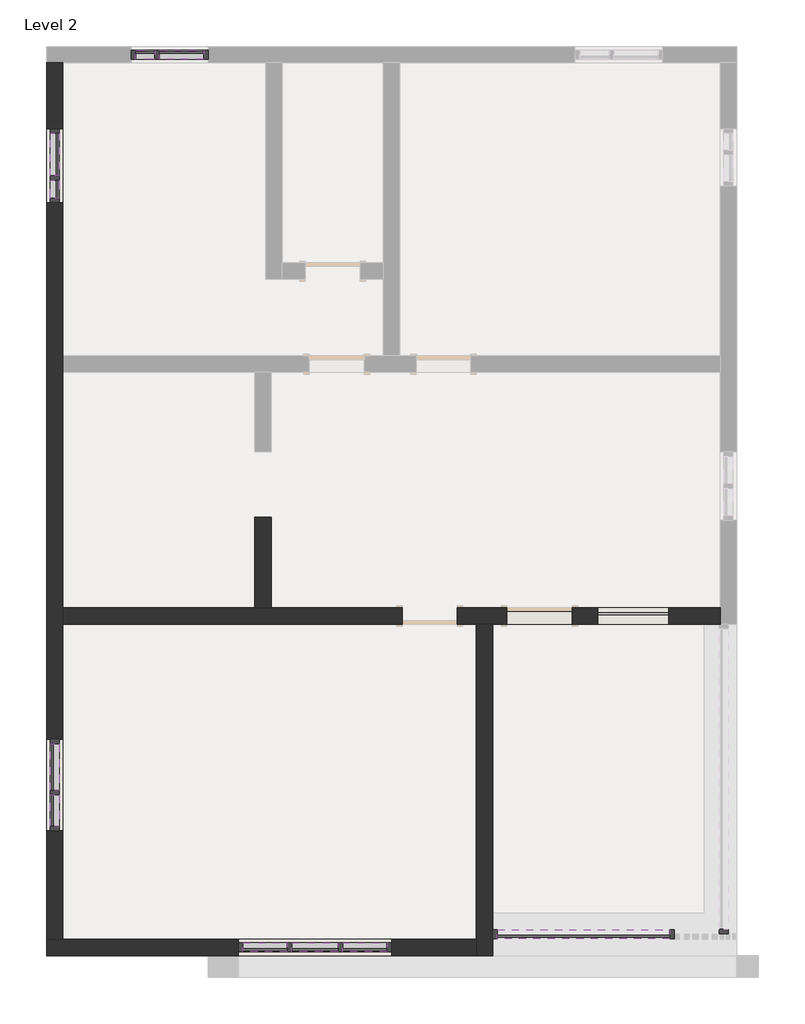
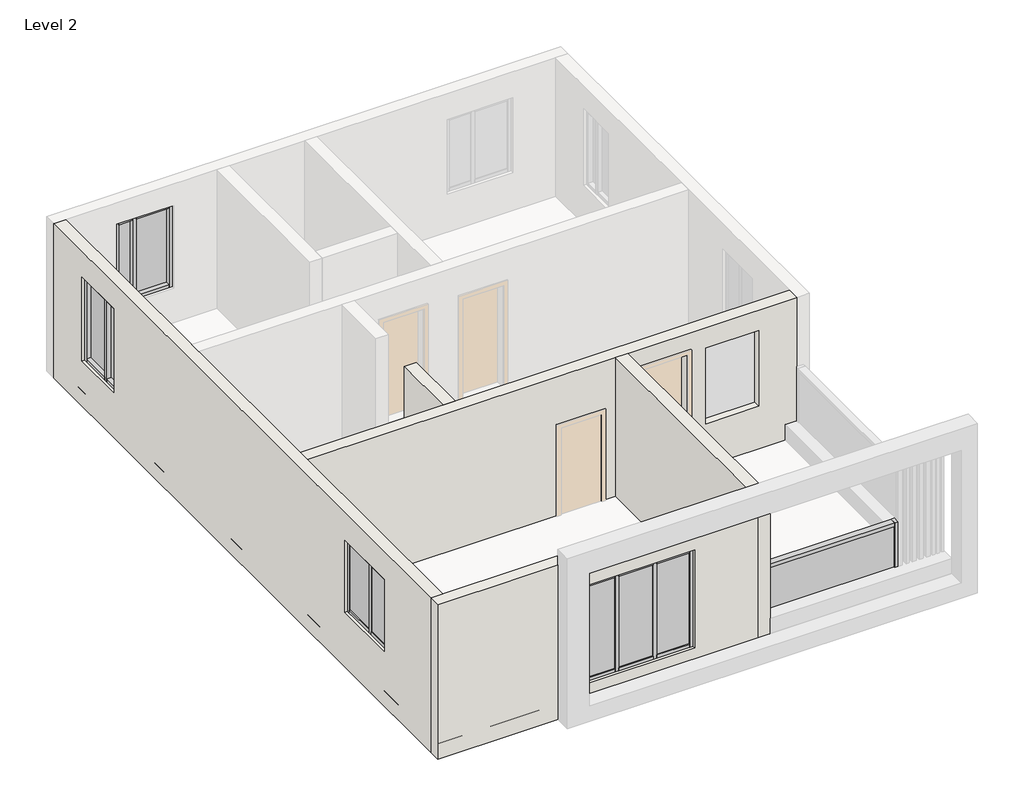
# One storey, part 1 of 2: 36 members, 10 plates, 5 walls.
"""IFC4 building model written with IfcOpenShell, lengths in millimetres."""

from ifc_helpers import new_model, si_unit, frame, origin, place, context, project, spatial, polyline, outline, extrude, faceted_brep, transform, mapped, element, save
from components import member_6fb4a552, member_e5d39754, member_3f0e0172, member_c304ec9f, member_9857a5fa, member_5215b92c, member_4adcbd6e, member_2f7568ae, member_e2524bce, member_4d06fd9b, member_4c0b5a72, member_ac37c43a, member_5cae1c76, member_8a84510b, member_26f0793c, member_c92b576d, member_86c371d5, member_6146d365, system_panel_glazed_d2c96357, system_panel_glazed_1c0d1104, system_panel_glazed_012e7337, system_panel_glazed_f6599d2c, system_panel_glazed_978b3bbc, system_panel_glazed_5a7f8ff5, system_panel_glazed_b38058b2, system_panel_glazed_fafcfa65, system_panel_glazed_51b229ca

model = new_model("IFC4")

# Units and contexts
model_context = context("Model", 3, world=origin())
ifc_project = project(units=[si_unit("LENGTHUNIT", "METRE", prefix="MILLI")], contexts=[model_context])

# Site, building, storey
site = spatial("IfcSite", under=ifc_project)
building = spatial("IfcBuilding", under=site)
storey = spatial("IfcBuildingStorey", under=building, Name="Level 2", Elevation=3048.0)

# Members
placement = place(None, origin())
member_shape = member_6fb4a552(model_context)
element("IfcMember", 1, ObjectType="Rectangular Mullion : 2.5\" x 5\" rectangular", at=placement, inside=storey, context=model_context, shape_type="MappedRepresentation", body=[
    mapped(member_shape, transform((-18412.7628107, -12019.2142965, 4124.9991955), x_axis=(0.0, 0.0, -1.0), y_axis=(1.0, 0.0, 0.0), z_axis=(0.0, -1.0, 0.0))),
])
member_2_shape = member_e5d39754(model_context)
element("IfcMember", 2, ObjectType="Rectangular Mullion : 2.5\" x 5\" rectangular", at=placement, inside=storey, context=model_context, shape_type="MappedRepresentation", body=[
    mapped(member_2_shape, transform((-18412.7628107, -2373.5642965, 3937.6338928), x_axis=(0.0, 0.0, -1.0), y_axis=(-1.0, 0.0, 0.0), z_axis=(0.0, 1.0, 0.0))),
])
element("IfcMember", 3, ObjectType="Rectangular Mullion : 2.5\" x 5\" rectangular", at=placement, inside=storey, context=model_context, shape_type="MappedRepresentation", body=[
    mapped(member_shape, transform((-18412.7628107, -11581.0642965, 5550.0097681), x_axis=(0.0, 0.0, 1.0), y_axis=(1.0, 0.0, 0.0), z_axis=(0.0, 1.0, 0.0))),
])
element("IfcMember", 4, ObjectType="Rectangular Mullion : 2.5\" x 5\" rectangular", at=placement, inside=storey, context=model_context, shape_type="MappedRepresentation", body=[
    mapped(member_2_shape, transform((-18412.7628107, -2964.1142965, 5597.0626061), x_axis=(0.0, 0.0, 1.0), y_axis=(-1.0, 0.0, 0.0), z_axis=(0.0, -1.0, 0.0))),
])
member_3_shape = member_3f0e0172(model_context)
element("IfcMember", 5, ObjectType="Rectangular Mullion : 2.5\" x 5\" rectangular", at=placement, inside=storey, context=model_context, shape_type="MappedRepresentation", body=[
    mapped(member_3_shape, transform((-14405.9128107, -13701.9642965, 5498.9031317), x_axis=(0.0, 0.0, 1.0), y_axis=(0.0, 1.0, 0.0), z_axis=(-1.0, 0.0, 0.0))),
])
element("IfcMember", 6, ObjectType="Rectangular Mullion : 2.5\" x 5\" rectangular", at=placement, inside=storey, context=model_context, shape_type="MappedRepresentation", body=[
    mapped(member_3_shape, transform((-15796.5628107, -13701.9642965, 5498.9031317), x_axis=(0.0, 0.0, 1.0), y_axis=(0.0, 1.0, 0.0), z_axis=(-1.0, 0.0, 0.0))),
])
element("IfcMember", 7, ObjectType="Rectangular Mullion : 2.5\" x 5\" rectangular", at=placement, inside=storey, context=model_context, shape_type="MappedRepresentation", body=[
    mapped(member_3_shape, transform((-16342.6628107, -1281.3642965, 5669.0676645), x_axis=(0.0, 0.0, 1.0), y_axis=(0.0, -1.0, 0.0), z_axis=(1.0, 0.0, 0.0))),
])
element("IfcMember", 8, ObjectType="Rectangular Mullion : 2.5\" x 5\" rectangular", at=placement, inside=storey, context=model_context, shape_type="MappedRepresentation", body=[
    mapped(member_3_shape, transform((-15180.6128107, -13701.9642965, 3567.7093947), x_axis=(0.0, 0.0, -1.0), y_axis=(0.0, 1.0, 0.0), z_axis=(1.0, 0.0, 0.0))),
])
element("IfcMember", 9, ObjectType="Rectangular Mullion : 2.5\" x 5\" rectangular", at=placement, inside=storey, context=model_context, shape_type="MappedRepresentation", body=[
    mapped(member_3_shape, transform((-13789.9628107, -13701.9642965, 3567.7093947), x_axis=(0.0, 0.0, -1.0), y_axis=(0.0, 1.0, 0.0), z_axis=(1.0, 0.0, 0.0))),
])
element("IfcMember", 10, ObjectType="Rectangular Mullion : 2.5\" x 5\" rectangular", at=placement, inside=storey, context=model_context, shape_type="MappedRepresentation", body=[
    mapped(member_3_shape, transform((-16958.6128107, -1281.3642965, 4034.7127427), x_axis=(0.0, 0.0, -1.0), y_axis=(0.0, -1.0, 0.0), z_axis=(-1.0, 0.0, 0.0))),
])
member_4_shape = member_c304ec9f(model_context)
element("IfcMember", 11, ObjectType="Rectangular Mullion : 2.5\" x 5\" rectangular", at=placement, inside=storey, context=model_context, shape_type="MappedRepresentation", body=[
    mapped(member_4_shape, transform((-15860.0628107, -13701.9642965, 3567.7093947), x_axis=(-1.0, 0.0, 0.0), y_axis=(0.0, 1.0, 0.0), z_axis=(0.0, 0.0, -1.0))),
])
element("IfcMember", 12, ObjectType="Rectangular Mullion : 2.5\" x 5\" rectangular", at=placement, inside=storey, context=model_context, shape_type="MappedRepresentation", body=[
    mapped(member_4_shape, transform((-13726.4628107, -13701.9642965, 5498.9031317), x_axis=(1.0, 0.0, 0.0), y_axis=(0.0, 1.0, 0.0), z_axis=(0.0, 0.0, 1.0))),
])
member_5_shape = member_9857a5fa(model_context)
element("IfcMember", 13, ObjectType="Rectangular Mullion : 2.5\" x 5\" rectangular", at=placement, inside=storey, context=model_context, shape_type="MappedRepresentation", body=[
    mapped(member_5_shape, transform((-15148.8628107, -13701.9642965, 3567.7093947), x_axis=(-1.0, 0.0, 0.0), y_axis=(0.0, 1.0, 0.0), z_axis=(0.0, 0.0, -1.0))),
])
element("IfcMember", 14, ObjectType="Rectangular Mullion : 2.5\" x 5\" rectangular", at=placement, inside=storey, context=model_context, shape_type="MappedRepresentation", body=[
    mapped(member_5_shape, transform((-14437.6628107, -13701.9642965, 3567.7093947), x_axis=(-1.0, 0.0, 0.0), y_axis=(0.0, 1.0, 0.0), z_axis=(0.0, 0.0, -1.0))),
])
member_6_shape = member_5215b92c(model_context)
element("IfcMember", 15, ObjectType="Rectangular Mullion : 2.5\" x 5\" rectangular", at=placement, inside=storey, context=model_context, shape_type="MappedRepresentation", body=[
    mapped(member_6_shape, transform((-15117.1128107, -13701.9642965, 5498.9031317), x_axis=(0.0, 0.0, 1.0), y_axis=(0.0, 1.0, 0.0), z_axis=(-1.0, 0.0, 0.0))),
])
element("IfcMember", 16, ObjectType="Rectangular Mullion : 2.5\" x 5\" rectangular", at=placement, inside=storey, context=model_context, shape_type="MappedRepresentation", body=[
    mapped(member_6_shape, transform((-18412.7628107, -10869.8642965, 5550.0097681), x_axis=(0.0, 0.0, 1.0), y_axis=(1.0, 0.0, 0.0), z_axis=(0.0, 1.0, 0.0))),
])
element("IfcMember", 17, ObjectType="Rectangular Mullion : 2.5\" x 5\" rectangular", at=placement, inside=storey, context=model_context, shape_type="MappedRepresentation", body=[
    mapped(member_6_shape, transform((-14469.4128107, -13701.9642965, 3567.7093947), x_axis=(0.0, 0.0, -1.0), y_axis=(0.0, 1.0, 0.0), z_axis=(1.0, 0.0, 0.0))),
])
element("IfcMember", 18, ObjectType="Rectangular Mullion : 2.5\" x 5\" rectangular", at=placement, inside=storey, context=model_context, shape_type="MappedRepresentation", body=[
    mapped(member_6_shape, transform((-18412.7628107, -11517.5642965, 4124.9991955), x_axis=(0.0, 0.0, -1.0), y_axis=(1.0, 0.0, 0.0), z_axis=(0.0, -1.0, 0.0))),
])
member_7_shape = member_4adcbd6e(model_context)
element("IfcMember", 19, ObjectType="Rectangular Mullion : 2.5\" x 5\" rectangular", at=placement, inside=storey, context=model_context, shape_type="MappedRepresentation", body=[
    mapped(member_7_shape, transform((-17022.1128107, -1281.3642965, 5669.0676645), x_axis=(0.0, 0.0, 1.0), y_axis=(0.0, -1.0, 0.0), z_axis=(1.0, 0.0, 0.0))),
])
member_8_shape = member_2f7568ae(model_context)
element("IfcMember", 20, ObjectType="Rectangular Mullion : 2.5\" x 5\" rectangular", at=placement, inside=storey, context=model_context, shape_type="MappedRepresentation", body=[
    mapped(member_8_shape, transform((-16990.3628107, -1281.3642965, 4034.7127427), x_axis=(1.0, 0.0, 0.0), y_axis=(0.0, -1.0, 0.0), z_axis=(0.0, 0.0, -1.0))),
])
element("IfcMember", 21, ObjectType="Rectangular Mullion : 2.5\" x 5\" rectangular", at=placement, inside=storey, context=model_context, shape_type="MappedRepresentation", body=[
    mapped(member_7_shape, transform((-17282.4628107, -1281.3642965, 4034.7127427), x_axis=(0.0, 0.0, -1.0), y_axis=(0.0, -1.0, 0.0), z_axis=(-1.0, 0.0, 0.0))),
])
member_9_shape = member_e2524bce(model_context)
element("IfcMember", 22, ObjectType="Rectangular Mullion : 2.5\" x 5\" rectangular", at=placement, inside=storey, context=model_context, shape_type="MappedRepresentation", body=[
    mapped(member_9_shape, transform((-17345.9628107, -1281.3642965, 5669.0676645), x_axis=(-1.0, 0.0, 0.0), y_axis=(0.0, -1.0, 0.0), z_axis=(0.0, 0.0, 1.0))),
])
element("IfcMember", 23, ObjectType="Rectangular Mullion : 2.5\" x 5\" rectangular", at=placement, inside=storey, context=model_context, shape_type="MappedRepresentation", body=[
    mapped(member_9_shape, transform((-16279.1628107, -1281.3642965, 4034.7127427), x_axis=(1.0, 0.0, 0.0), y_axis=(0.0, -1.0, 0.0), z_axis=(0.0, 0.0, -1.0))),
])
member_10_shape = member_4d06fd9b(model_context)
element("IfcMember", 24, ObjectType="Rectangular Mullion : 2.5\" x 5\" rectangular", at=placement, inside=storey, context=model_context, shape_type="MappedRepresentation", body=[
    mapped(member_10_shape, transform((-18412.7628107, -3275.2642965, 5597.0626061), x_axis=(0.0, 0.0, 1.0), y_axis=(-1.0, 0.0, 0.0), z_axis=(0.0, -1.0, 0.0))),
])
member_11_shape = member_4c0b5a72(model_context)
element("IfcMember", 25, ObjectType="Rectangular Mullion : 2.5\" x 5\" rectangular", at=placement, inside=storey, context=model_context, shape_type="MappedRepresentation", body=[
    mapped(member_11_shape, transform((-18412.7628107, -2995.8642965, 3937.6338928), x_axis=(0.0, -1.0, 0.0), y_axis=(-1.0, 0.0, 0.0), z_axis=(0.0, 0.0, -1.0))),
])
element("IfcMember", 26, ObjectType="Rectangular Mullion : 2.5\" x 5\" rectangular", at=placement, inside=storey, context=model_context, shape_type="MappedRepresentation", body=[
    mapped(member_10_shape, transform((-18412.7628107, -3027.6142965, 3937.6338928), x_axis=(0.0, 0.0, -1.0), y_axis=(-1.0, 0.0, 0.0), z_axis=(0.0, 1.0, 0.0))),
])
member_12_shape = member_ac37c43a(model_context)
element("IfcMember", 27, ObjectType="Rectangular Mullion : 2.5\" x 5\" rectangular", at=placement, inside=storey, context=model_context, shape_type="MappedRepresentation", body=[
    mapped(member_12_shape, transform((-18412.7628107, -3338.7642965, 3937.6338928), x_axis=(0.0, -1.0, 0.0), y_axis=(-1.0, 0.0, 0.0), z_axis=(0.0, 0.0, -1.0))),
])
element("IfcMember", 28, ObjectType="Rectangular Mullion : 2.5\" x 5\" rectangular", at=placement, inside=storey, context=model_context, shape_type="MappedRepresentation", body=[
    mapped(member_12_shape, transform((-18412.7628107, -2310.0642965, 5597.0626061), x_axis=(0.0, 1.0, 0.0), y_axis=(-1.0, 0.0, 0.0), z_axis=(0.0, 0.0, 1.0))),
])
member_13_shape = member_5cae1c76(model_context)
element("IfcMember", 29, ObjectType="Rectangular Mullion : 2.5\" x 5\" rectangular", at=placement, inside=storey, context=model_context, shape_type="MappedRepresentation", body=[
    mapped(member_13_shape, transform((-18412.7628107, -11549.3142965, 4124.9991955), x_axis=(0.0, 1.0, 0.0), y_axis=(1.0, 0.0, 0.0), z_axis=(0.0, 0.0, -1.0))),
])
member_14_shape = member_8a84510b(model_context)
element("IfcMember", 30, ObjectType="Rectangular Mullion : 2.5\" x 5\" rectangular", at=placement, inside=storey, context=model_context, shape_type="MappedRepresentation", body=[
    mapped(member_14_shape, transform((-18412.7628107, -12082.7142965, 5550.0097681), x_axis=(0.0, -1.0, 0.0), y_axis=(1.0, 0.0, 0.0), z_axis=(0.0, 0.0, 1.0))),
])
element("IfcMember", 31, ObjectType="Rectangular Mullion : 2.5\" x 5\" rectangular", at=placement, inside=storey, context=model_context, shape_type="MappedRepresentation", body=[
    mapped(member_14_shape, transform((-18412.7628107, -10806.3642965, 4124.9991955), x_axis=(0.0, 1.0, 0.0), y_axis=(1.0, 0.0, 0.0), z_axis=(0.0, 0.0, -1.0))),
])
member_15_shape = member_26f0793c(model_context)
element("IfcMember", 32, ObjectType="Rectangular Mullion : 2.5\" x 5\" rectangular", at=placement, inside=storey, context=model_context, shape_type="MappedRepresentation", body=[
    mapped(member_15_shape, transform((-12316.7628107, -13518.1585678, 3513.341316), x_axis=(-1.0, 0.0, 0.0), y_axis=(0.0, 1.0, 0.0), z_axis=(0.0, 0.0, -1.0))),
])
member_16_shape = member_c92b576d(model_context)
element("IfcMember", 33, ObjectType="Rectangular Mullion : 2.5\" x 5\" rectangular", at=placement, inside=storey, context=model_context, shape_type="MappedRepresentation", body=[
    mapped(member_16_shape, transform((-12253.2628107, -13518.1585678, 4533.6270977), x_axis=(0.0, 0.0, 1.0), y_axis=(0.0, 1.0, 0.0), z_axis=(-1.0, 0.0, 0.0))),
])
element("IfcMember", 34, ObjectType="Rectangular Mullion : 2.5\" x 5\" rectangular", at=placement, inside=storey, context=model_context, shape_type="MappedRepresentation", body=[
    mapped(member_15_shape, transform((-9791.4069383, -13518.1585678, 4533.6270977), x_axis=(1.0, 0.0, 0.0), y_axis=(0.0, 1.0, 0.0), z_axis=(0.0, 0.0, 1.0))),
])
member_17_shape = member_86c371d5(model_context)
element("IfcMember", 35, ObjectType="Rectangular Mullion : 2.5\" x 5\" rectangular", at=placement, inside=storey, context=model_context, shape_type="MappedRepresentation", body=[
    mapped(member_17_shape, transform((-9103.6628107, -13447.9642965, 3436.1535444), x_axis=(0.0, 0.0, -1.0), y_axis=(1.0, 0.0, 0.0), z_axis=(0.0, -1.0, 0.0))),
])
member_18_shape = member_6146d365(model_context)
element("IfcMember", 36, ObjectType="Rectangular Mullion : 2.5\" x 5\" rectangular", at=placement, inside=storey, context=model_context, shape_type="MappedRepresentation", body=[
    mapped(member_18_shape, transform((-9103.6628107, -13511.4642965, 4732.9155045), x_axis=(0.0, -1.0, 0.0), y_axis=(1.0, 0.0, 0.0), z_axis=(0.0, 0.0, 1.0))),
])

# Plates
system_panel_glazed_shape = system_panel_glazed_d2c96357(model_context)
element("IfcPlate", 37, ObjectType="System Panel : Glazed", at=placement, inside=storey, context=model_context, shape_type="MappedRepresentation", body=[
    mapped(system_panel_glazed_shape, transform((-14793.2628107, -13701.9642965, 3631.2093947), x_axis=(-1.0, 0.0, 0.0), y_axis=(0.0, -1.0, 0.0), z_axis=(0.0, 0.0, 1.0))),
])
system_panel_glazed_2_shape = system_panel_glazed_1c0d1104(model_context)
element("IfcPlate", 38, ObjectType="System Panel : Glazed", at=placement, inside=storey, context=model_context, shape_type="MappedRepresentation", body=[
    mapped(system_panel_glazed_2_shape, transform((-14097.9378107, -13701.9642965, 3631.2093947), x_axis=(-1.0, 0.0, 0.0), y_axis=(0.0, -1.0, 0.0), z_axis=(0.0, 0.0, 1.0))),
])
element("IfcPlate", 39, ObjectType="System Panel : Glazed", at=placement, inside=storey, context=model_context, shape_type="MappedRepresentation", body=[
    mapped(system_panel_glazed_2_shape, transform((-15488.5878107, -13701.9642965, 3631.2093947), x_axis=(-1.0, 0.0, 0.0), y_axis=(0.0, -1.0, 0.0), z_axis=(0.0, 0.0, 1.0))),
])
system_panel_glazed_3_shape = system_panel_glazed_012e7337(model_context)
element("IfcPlate", 40, ObjectType="System Panel : Glazed", at=placement, inside=storey, context=model_context, shape_type="MappedRepresentation", body=[
    mapped(system_panel_glazed_3_shape, transform((-17152.2878107, -1281.3642965, 4098.2127427), x_axis=(1.0, 0.0, 0.0), y_axis=(0.0, 1.0, 0.0), z_axis=(0.0, 0.0, 1.0))),
])
system_panel_glazed_4_shape = system_panel_glazed_f6599d2c(model_context)
element("IfcPlate", 41, ObjectType="System Panel : Glazed", at=placement, inside=storey, context=model_context, shape_type="MappedRepresentation", body=[
    mapped(system_panel_glazed_4_shape, transform((-16650.6378107, -1281.3642965, 4098.2127427), x_axis=(1.0, 0.0, 0.0), y_axis=(0.0, 1.0, 0.0), z_axis=(0.0, 0.0, 1.0))),
])
system_panel_glazed_5_shape = system_panel_glazed_978b3bbc(model_context)
element("IfcPlate", 42, ObjectType="System Panel : Glazed", at=placement, inside=storey, context=model_context, shape_type="MappedRepresentation", body=[
    mapped(system_panel_glazed_5_shape, transform((-18412.7628107, -2668.8392965, 4001.1338928), x_axis=(0.0, -1.0, 0.0), y_axis=(1.0, 0.0, 0.0), z_axis=(0.0, 0.0, 1.0))),
])
system_panel_glazed_6_shape = system_panel_glazed_5a7f8ff5(model_context)
element("IfcPlate", 43, ObjectType="System Panel : Glazed", at=placement, inside=storey, context=model_context, shape_type="MappedRepresentation", body=[
    mapped(system_panel_glazed_6_shape, transform((-18412.7628107, -3151.4392965, 4001.1338928), x_axis=(0.0, -1.0, 0.0), y_axis=(1.0, 0.0, 0.0), z_axis=(0.0, 0.0, 1.0))),
])
system_panel_glazed_7_shape = system_panel_glazed_b38058b2(model_context)
element("IfcPlate", 44, ObjectType="System Panel : Glazed", at=placement, inside=storey, context=model_context, shape_type="MappedRepresentation", body=[
    mapped(system_panel_glazed_7_shape, transform((-18412.7628107, -11800.1392965, 4188.4991955), x_axis=(0.0, 1.0, 0.0), y_axis=(-1.0, 0.0, 0.0), z_axis=(0.0, 0.0, 1.0))),
])
system_panel_glazed_8_shape = system_panel_glazed_fafcfa65(model_context)
element("IfcPlate", 45, ObjectType="System Panel : Glazed", at=placement, inside=storey, context=model_context, shape_type="MappedRepresentation", body=[
    mapped(system_panel_glazed_8_shape, transform((-18412.7628107, -11193.7142965, 4188.4991955), x_axis=(0.0, 1.0, 0.0), y_axis=(-1.0, 0.0, 0.0), z_axis=(0.0, 0.0, 1.0))),
])
system_panel_glazed_9_shape = system_panel_glazed_51b229ca(model_context)
element("IfcPlate", 46, ObjectType="System Panel : Glazed", at=placement, inside=storey, context=model_context, shape_type="MappedRepresentation", body=[
    mapped(system_panel_glazed_9_shape, transform((-11054.0848745, -13518.1585678, 3513.341316), x_axis=(-1.0, 0.0, 0.0), y_axis=(0.0, -1.0, 0.0), z_axis=(0.0, 0.0, 1.0))),
])

# Walls
element("IfcWall", 47, ObjectType="9\"", at=placement, inside=storey, context=model_context, shape_type="Brep", body=[
    faceted_brep([(-18298.4628107, -8977.5642965, 6096.0), (-15631.4628107, -8977.5642965, 6096.0), (-15402.8628107, -8977.5642965, 6096.0), (-9154.4628107, -8977.5642965, 6096.0), (-9154.4628107, -8977.5642965, 3048.0), (-12812.0628107, -8977.5642965, 3048.0), (-12812.0628107, -8977.5642965, 5080.0), (-13574.0628107, -8977.5642965, 5080.0), (-13574.0628107, -8977.5642965, 3048.0), (-15402.8628107, -8977.5642965, 3048.0), (-15631.4628107, -8977.5642965, 3048.0), (-18298.4628107, -8977.5642965, 3048.0), (-12126.2628107, -8977.5642965, 3556.0), (-11211.8628107, -8977.5642965, 3556.0), (-11211.8628107, -8977.5642965, 5689.6), (-12126.2628107, -8977.5642965, 5689.6), (-10856.2628107, -8977.5642965, 5688.4188539), (-10856.2628107, -8977.5642965, 4193.7740011), (-9865.6628107, -8977.5642965, 4193.7740011), (-9865.6628107, -8977.5642965, 5688.4188539), (-9154.4628107, -9206.1642965, 6096.0), (-12316.7628107, -9206.1642965, 6096.0), (-12545.3628107, -9206.1642965, 6096.0), (-18298.4628107, -9206.1642965, 6096.0), (-18298.4628107, -9206.1642965, 3048.0), (-13574.0628107, -9206.1642965, 3048.0), (-13574.0628107, -9206.1642965, 5080.0), (-12812.0628107, -9206.1642965, 5080.0), (-12812.0628107, -9206.1642965, 3048.0), (-12545.3628107, -9206.1642965, 3048.0), (-12316.7628107, -9206.1642965, 3048.0), (-9154.4628107, -9206.1642965, 3048.0), (-11211.8628107, -9206.1642965, 3556.0), (-12126.2628107, -9206.1642965, 3556.0), (-12126.2628107, -9206.1642965, 5689.6), (-11211.8628107, -9206.1642965, 5689.6), (-10856.2628107, -9206.1642965, 4193.7740011), (-10856.2628107, -9206.1642965, 5688.4188539), (-9865.6628107, -9206.1642965, 5688.4188539), (-9865.6628107, -9206.1642965, 4193.7740011)], [[[0, 1, 2, 3, 4, 5, 6, 7, 8, 9, 10, 11], [12, 13, 14, 15], [16, 17, 18, 19]], [[20, 21, 22, 23, 24, 25, 26, 27, 28, 29, 30, 31], [32, 33, 34, 35], [36, 37, 38, 39]], [[4, 31, 30, 29, 28, 5]], [[24, 11, 10, 9, 8, 25]], [[3, 2, 1, 0, 23, 22, 21, 20]], [[4, 3, 20, 31]], [[0, 11, 24, 23]], [[33, 32, 13, 12]], [[34, 33, 12, 15]], [[35, 34, 15, 14]], [[32, 35, 14, 13]], [[26, 25, 8, 7]], [[27, 26, 7, 6]], [[28, 27, 6, 5]], [[36, 17, 16, 37]], [[37, 16, 19, 38]], [[38, 19, 18, 39]], [[17, 36, 39, 18]]]),
])
element("IfcWall", 48, ObjectType="9\"", at=placement, inside=storey, context=model_context, shape_type="Brep", body=[
    faceted_brep([(-12545.3628107, -9206.1642965, 3048.0), (-12545.3628107, -13587.6642965, 3048.0), (-12545.3628107, -13816.2642965, 3048.0), (-12545.3628107, -13816.2642965, 6096.0), (-12545.3628107, -13587.6642965, 6096.0), (-12545.3628107, -9206.1642965, 6096.0), (-12316.7628107, -9206.1642965, 3048.0), (-12316.7628107, -9206.1642965, 6096.0), (-12316.7628107, -13816.2642965, 6096.0), (-12316.7628107, -13816.2642965, 3048.0)], [[[0, 1, 2, 3, 4, 5]], [[6, 7, 8, 9]], [[2, 1, 0, 6, 9]], [[5, 4, 3, 8, 7]], [[0, 5, 7, 6]], [[3, 2, 9, 8]]]),
])
element("IfcWall", 49, ObjectType="9\"", at=placement, inside=storey, context=model_context, shape_type="Brep", body=[
    faceted_brep([(-12545.3628107, -13587.6642965, 3048.0), (-18298.4628107, -13587.6642965, 3048.0), (-18527.0628107, -13587.6642965, 3048.0), (-18527.0628107, -13587.6642965, 6096.0), (-18298.4628107, -13587.6642965, 6096.0), (-12545.3628107, -13587.6642965, 6096.0), (-13726.4628107, -13587.6642965, 3567.7093947), (-13726.4628107, -13587.6642965, 5498.9031317), (-15860.0628107, -13587.6642965, 5498.9031317), (-15860.0628107, -13587.6642965, 3567.7093947), (-18527.0628107, -13816.2642965, 3048.0), (-12545.3628107, -13816.2642965, 3048.0), (-12545.3628107, -13816.2642965, 6096.0), (-18527.0628107, -13816.2642965, 6096.0), (-13726.4628107, -13816.2642965, 5498.9031317), (-13726.4628107, -13816.2642965, 3567.7093947), (-15860.0628107, -13816.2642965, 3567.7093947), (-15860.0628107, -13816.2642965, 5498.9031317)], [[[0, 1, 2, 3, 4, 5], [6, 7, 8, 9]], [[10, 11, 12, 13], [14, 15, 16, 17]], [[2, 1, 0, 11, 10]], [[5, 4, 3, 13, 12]], [[0, 5, 12, 11]], [[3, 2, 10, 13]], [[6, 15, 14, 7]], [[7, 14, 17, 8]], [[8, 17, 16, 9]], [[15, 6, 9, 16]]]),
])
element("IfcWall", 50, ObjectType="9\"", at=placement, inside=storey, context=model_context, shape_type="Brep", body=[
    faceted_brep([(-18527.0628107, -1395.6642965, 3048.0), (-18527.0628107, -13587.6642965, 3048.0), (-18527.0628107, -13587.6642965, 6096.0), (-18527.0628107, -1395.6642965, 6096.0), (-18527.0628107, -2310.0642965, 3937.6338928), (-18527.0628107, -2310.0642965, 5597.0626061), (-18527.0628107, -3338.7642965, 5597.0626061), (-18527.0628107, -3338.7642965, 3937.6338928), (-18527.0628107, -12082.7142965, 5550.0097681), (-18527.0628107, -12082.7142965, 4124.9991955), (-18527.0628107, -10806.3642965, 4124.9991955), (-18527.0628107, -10806.3642965, 5550.0097681), (-18298.4628107, -13587.6642965, 3048.0), (-18298.4628107, -9206.1642965, 3048.0), (-18298.4628107, -8977.5642965, 3048.0), (-18298.4628107, -5700.9642965, 3048.0), (-18298.4628107, -5472.3642965, 3048.0), (-18298.4628107, -1395.6642965, 3048.0), (-18298.4628107, -1395.6642965, 6096.0), (-18298.4628107, -5472.3642965, 6096.0), (-18298.4628107, -5700.9642965, 6096.0), (-18298.4628107, -8977.5642965, 6096.0), (-18298.4628107, -9206.1642965, 6096.0), (-18298.4628107, -13587.6642965, 6096.0), (-18298.4628107, -2310.0642965, 5597.0626061), (-18298.4628107, -2310.0642965, 3937.6338928), (-18298.4628107, -3338.7642965, 3937.6338928), (-18298.4628107, -3338.7642965, 5597.0626061), (-18298.4628107, -12082.7142965, 4124.9991955), (-18298.4628107, -12082.7142965, 5550.0097681), (-18298.4628107, -10806.3642965, 5550.0097681), (-18298.4628107, -10806.3642965, 4124.9991955)], [[[0, 1, 2, 3], [4, 5, 6, 7], [8, 9, 10, 11]], [[12, 13, 14, 15, 16, 17, 18, 19, 20, 21, 22, 23], [24, 25, 26, 27], [28, 29, 30, 31]], [[1, 0, 17, 16, 15, 14, 13, 12]], [[3, 2, 23, 22, 21, 20, 19, 18]], [[0, 3, 18, 17]], [[2, 1, 12, 23]], [[24, 5, 4, 25]], [[5, 24, 27, 6]], [[6, 27, 26, 7]], [[25, 4, 7, 26]], [[28, 9, 8, 29]], [[29, 8, 11, 30]], [[30, 11, 10, 31]], [[9, 28, 31, 10]]]),
])
element("IfcWall", 51, ObjectType="9\"", at=placement, inside=storey, context=model_context, shape_type="SweptSolid", body=[
    extrude(outline(polyline([(-15631.4628107, -8977.5642965), (-15631.4628107, -7720.2642965), (-15402.8628107, -7720.2642965), (-15402.8628107, -8977.5642965), (-15631.4628107, -8977.5642965)])), frame((0.0, 0.0, 3048.0), z_axis=(0.0, 0.0, 1.0), x_axis=(1.0, 0.0, 0.0)), (0.0, 0.0, 1.0), 3048.0),
])

save(model, "model.ifc")

# Revit data of these elements
# Type "Rectangular Mullion : 2.5\" x 5\" rectangular"
#   built-in parameter 1007304 = 0.416667 (stored number, unit not read)
#   built-in parameter 1007301 = 0.104167 (stored number, unit not read)
#   built-in parameter 1007300 = 0.104167 (stored number, unit not read)
# Type "System Panel : Glazed"
#   Construction Type Id = "GSP4R"
#   Analytic Construction = "1/8 in Pilkington single glazing"
#   Visual Light Transmittance = 0.9
#   Solar Heat Gain Coefficient = 0.86
#   Heat Transfer Coefficient (U) = 1.18115 BTU/(h·ft²·°F)
#   Define Thermal Properties by = 1
# Type "9\""
#   Assembly Code = "B2010"
#   Layers, outside or top first: 0' - 9" no material (function 1)
# Elements 1, 2, 3, 4, 5, 6, 7, 8, 9, 10, 11, 12, 13, 14, 15, 16, 17, 18, 19, 20, 21, 22, 23, 24, 25, 26, 27, 28, 29, 30, 31, 32, 33, 34, 35, 36 (IfcMember, "Rectangular Mullion : 2.5\" x 5\" rectangular")
#   Phase Created = New Construction
#   Materials on its faces: "Aluminum"
# Elements 37, 38, 39, 40, 41, 42, 43, 44, 45, 46 (IfcPlate, "System Panel : Glazed")
#   Phase Created = New Construction
#   Materials on its faces: "Glass"
# Elements 47, 48, 49, 50, 51 (IfcWall, "9\"")
#   Top Offset = 0' - 0"
#   Base Offset = 0' - 0"
#   Unconnected Height = 10' - 0"
#   wall height = 10' - 0"
#   Phase Created = New Construction
#   Base Constraint = Level 2
#   Materials on its faces: "Default Wall"
# Materials
#   "Aluminum": class "Metal", colour RGB 247 247 247, transparency 0, Description = "Aluminum 6061", Cost = 0
#   "Glass": class "Glass", colour RGB 0 128 192, transparency 0.75, Description = "Soda Lime Glass", Cost = 0
#   "Default Wall": colour RGB 128 128 128, transparency 0, Cost = 0
